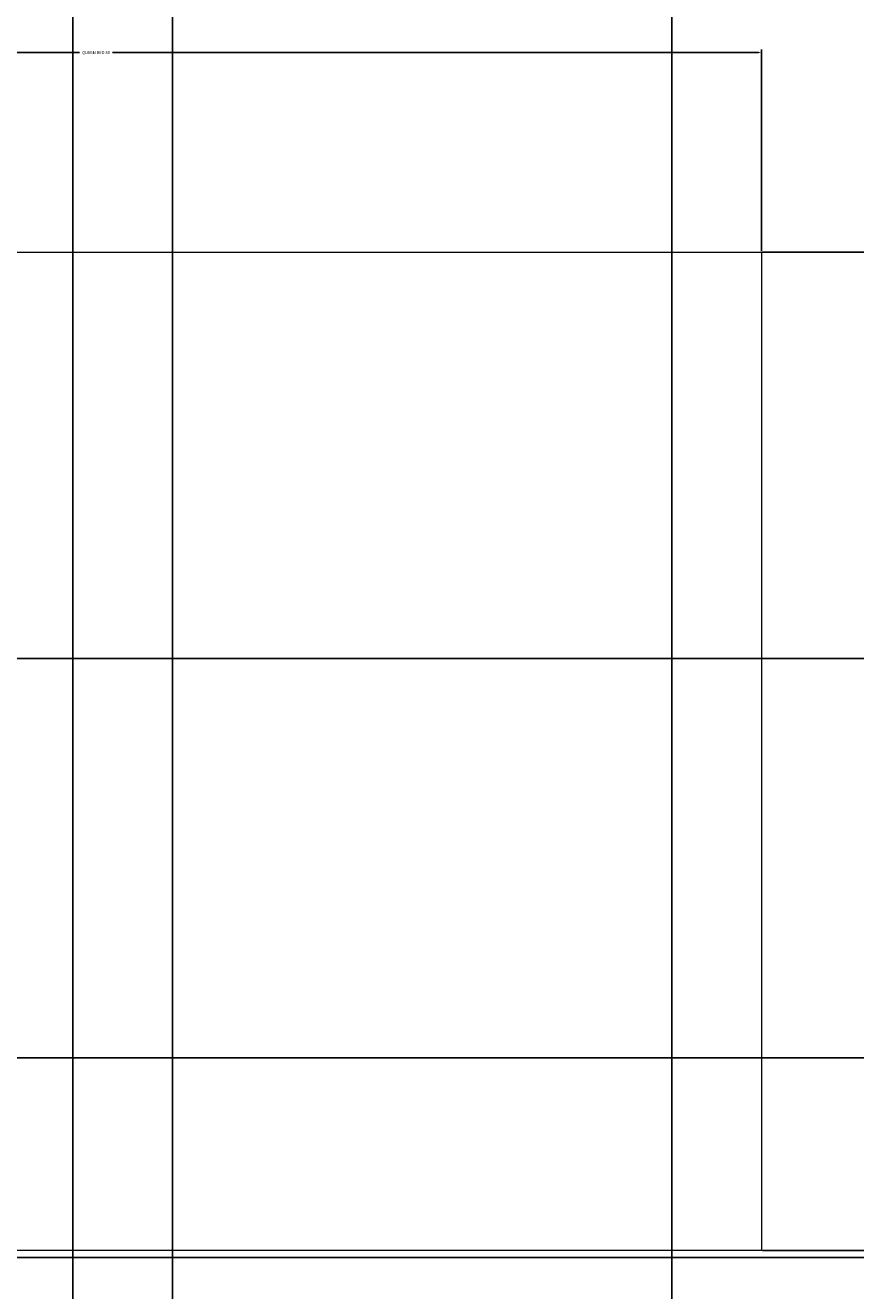
# Model space of a CAD drawing. Units: inches. Extents: x 2231 to 2461, y 2045 to 2455.
# Tile 73 of 95: x 2296 to 2346, y 2333 to 2409. Entities that reach past the tile are written whole.
import ezdxf

# ---------------------------------------------------------------- set-up
doc = ezdxf.new("R2010")
doc.units = ezdxf.units.IN
doc.layers.add('A-ANNO-DIMS', color=2, linetype='Continuous', lineweight=18)
doc.layers.add('A-FURN', color=9, linetype='Continuous', lineweight=18)
doc.styles.get("Standard").update_dxf_attribs({"font": 'arial.ttf'})
doc.dimstyles.get("Standard").update_dxf_attribs({"dimtxt": 0.18, "dimasz": 0.18, "dimexe": 0.18, "dimexo": 0.0625, "dimgap": 0.09, "dimtad": 0, "dimtih": 1, "dimtoh": 1, "dimdec": 4, "dimzin": 0, "dimdsep": 46, "dimtxsty": 'Standard', "dimcen": 0.09, "dimadec": 0, "dimazin": 0, "dimtfac": 1, "dimtdec": 4, "dimtofl": 0, "dimtmove": 0, "dimatfit": 3, "dimfxl": 1, "dimtolj": 1, "dimtzin": 0, "dimarcsym": 0})

# ---------------------------------------------------------------- blocks, each defined once
blk = doc.blocks.new('Bed - Queen')
for p, q in [((0, -80.00003), (0, 0)), ((59.99999, 0), (59.99999, -80.00003)), ((59.99999, -80.00003), (0, -80.00003))]:
    blk.add_line(p, q)
blk = doc.blocks.new('*D19')
at = {"layer": 'A-ANNO-DIMS', "color": 0, "lineweight": -2, "transparency": 16777216}
for p, q in [((2260.188, 2395.316), (2260.188, 2407.433)), ((2260.368, 2407.253), (2299.194, 2407.253)), ((2340.008, 2407.253), (2301.182, 2407.253)), ((2340.188, 2395.316), (2340.188, 2407.433))]:
    blk.add_line(p, q, dxfattribs=at)
at = {"layer": 'A-ANNO-DIMS', "color": 0, "transparency": 16777216}
for points in [[(2260.368, 2407.283), (2260.368, 2407.223), (2260.188, 2407.253)], [(2340.008, 2407.283), (2340.008, 2407.223), (2340.188, 2407.253)]]:
    blk.add_solid(points, dxfattribs=at)
at = {"layer": 'Defpoints', "color": 0, "transparency": 16777216}
for p in [(2260.188, 2407.253), (2260.188, 2395.253), (2340.188, 2395.253)]:
    blk.add_point(p, dxfattribs=at)
at = {"layer": 'A-ANNO-DIMS', "color": 0, "transparency": 16777216, "insert": (2300.188, 2407.253), "char_height": 0.18, "attachment_point": 5}
blk.add_mtext('\\A1;QUEEN BED 80', dxfattribs=at)
blk = doc.blocks.new('*D20')
at = {"layer": 'A-ANNO-DIMS', "color": 0, "lineweight": -2, "transparency": 16777216}
for p, q in [((2340.251, 2395.253), (2352.368, 2395.253)), ((2352.188, 2395.073), (2352.188, 2365.435)), ((2352.188, 2335.433), (2352.188, 2365.071)), ((2340.251, 2335.253), (2352.368, 2335.253))]:
    blk.add_line(p, q, dxfattribs=at)
at = {"layer": 'A-ANNO-DIMS', "color": 0, "transparency": 16777216}
for points in [[(2352.158, 2395.073), (2352.218, 2395.073), (2352.188, 2395.253)], [(2352.158, 2335.433), (2352.218, 2335.433), (2352.188, 2335.253)]]:
    blk.add_solid(points, dxfattribs=at)
at = {"layer": 'Defpoints', "color": 0, "transparency": 16777216}
for p in [(2340.188, 2395.253), (2352.188, 2395.253), (2340.188, 2335.253)]:
    blk.add_point(p, dxfattribs=at)
at = {"layer": 'A-ANNO-DIMS', "color": 0, "transparency": 16777216, "insert": (2352.188, 2365.253), "char_height": 0.18, "attachment_point": 5}
blk.add_mtext('\\A1;60', dxfattribs=at)
blk = doc.blocks.new('*D49')
at = {"layer": 'A-ANNO-DIMS', "color": 0, "lineweight": -2, "transparency": 16777216}
for p, q in [((2298.794, 2182.895), (2298.794, 2454.645)), ((2298.974, 2454.465), (2301.644, 2454.465)), ((2304.614, 2454.465), (2301.943, 2454.465)), ((2304.794, 2182.895), (2304.794, 2454.645))]:
    blk.add_line(p, q, dxfattribs=at)
at = {"layer": 'A-ANNO-DIMS', "color": 0, "transparency": 16777216}
for points in [[(2298.974, 2454.495), (2298.974, 2454.435), (2298.794, 2454.465)], [(2304.614, 2454.495), (2304.614, 2454.435), (2304.794, 2454.465)]]:
    blk.add_solid(points, dxfattribs=at)
at = {"layer": 'Defpoints', "color": 0, "transparency": 16777216}
for p in [(2304.794, 2454.465), (2298.794, 2182.833), (2304.794, 2182.833)]:
    blk.add_point(p, dxfattribs=at)
at = {"layer": 'A-ANNO-DIMS', "color": 0, "transparency": 16777216, "insert": (2301.794, 2454.465), "char_height": 0.18, "attachment_point": 5}
blk.add_mtext('\\A1;6', dxfattribs=at)
blk = doc.blocks.new('*D50')
at = {"layer": 'A-ANNO-DIMS', "color": 0, "lineweight": -2, "transparency": 16777216}
for p, q in [((2304.794, 2182.895), (2304.794, 2454.645)), ((2304.974, 2454.465), (2319.575, 2454.465)), ((2334.614, 2454.465), (2320.012, 2454.465)), ((2334.794, 2182.895), (2334.794, 2454.645))]:
    blk.add_line(p, q, dxfattribs=at)
at = {"layer": 'A-ANNO-DIMS', "color": 0, "transparency": 16777216}
for points in [[(2304.974, 2454.495), (2304.974, 2454.435), (2304.794, 2454.465)], [(2334.614, 2454.495), (2334.614, 2454.435), (2334.794, 2454.465)]]:
    blk.add_solid(points, dxfattribs=at)
at = {"layer": 'Defpoints', "color": 0, "transparency": 16777216}
for p in [(2334.794, 2454.465), (2304.794, 2182.833), (2334.794, 2182.833)]:
    blk.add_point(p, dxfattribs=at)
at = {"layer": 'A-ANNO-DIMS', "color": 0, "transparency": 16777216, "insert": (2319.794, 2454.465), "char_height": 0.18, "attachment_point": 5}
blk.add_mtext('\\A1;30', dxfattribs=at)
blk = doc.blocks.new('*D53')
at = {"layer": 'A-ANNO-DIMS', "color": 0, "lineweight": -2, "transparency": 16777216}
for p, q in [((2372.731, 2346.833), (2230.981, 2346.833)), ((2231.161, 2346.653), (2231.161, 2341.013)), ((2231.161, 2335.013), (2231.161, 2340.652)), ((2372.731, 2334.833), (2230.981, 2334.833))]:
    blk.add_line(p, q, dxfattribs=at)
at = {"layer": 'A-ANNO-DIMS', "color": 0, "transparency": 16777216}
for points in [[(2231.131, 2346.653), (2231.191, 2346.653), (2231.161, 2346.833)], [(2231.131, 2335.013), (2231.191, 2335.013), (2231.161, 2334.833)]]:
    blk.add_solid(points, dxfattribs=at)
at = {"layer": 'Defpoints', "color": 0, "transparency": 16777216}
for p in [(2231.161, 2346.833), (2372.794, 2346.833), (2372.794, 2334.833)]:
    blk.add_point(p, dxfattribs=at)
at = {"layer": 'A-ANNO-DIMS', "color": 0, "transparency": 16777216, "insert": (2231.161, 2340.833), "char_height": 0.18, "attachment_point": 5}
blk.add_mtext('\\A1;12', dxfattribs=at)
blk = doc.blocks.new('*D54')
at = {"layer": 'A-ANNO-DIMS', "color": 0, "lineweight": -2, "transparency": 16777216}
for p, q in [((2372.731, 2370.833), (2230.981, 2370.833)), ((2231.161, 2370.653), (2231.161, 2359.013)), ((2231.161, 2347.013), (2231.161, 2358.652)), ((2372.731, 2346.833), (2230.981, 2346.833))]:
    blk.add_line(p, q, dxfattribs=at)
at = {"layer": 'A-ANNO-DIMS', "color": 0, "transparency": 16777216}
for points in [[(2231.131, 2370.653), (2231.191, 2370.653), (2231.161, 2370.833)], [(2231.131, 2347.013), (2231.191, 2347.013), (2231.161, 2346.833)]]:
    blk.add_solid(points, dxfattribs=at)
at = {"layer": 'Defpoints', "color": 0, "transparency": 16777216}
for p in [(2231.161, 2370.833), (2372.794, 2370.833), (2372.794, 2346.833)]:
    blk.add_point(p, dxfattribs=at)
at = {"layer": 'A-ANNO-DIMS', "color": 0, "transparency": 16777216, "insert": (2231.161, 2358.833), "char_height": 0.18, "attachment_point": 5}
blk.add_mtext('\\A1;24', dxfattribs=at)

msp = doc.modelspace()

# ---------------------------------------------------------------- block references
at = {"layer": 'A-FURN', "rotation": 90}
msp.add_blockref('Bed - Queen', (2260.1881, 2335.2534), dxfattribs=at)

# ---------------------------------------------------------------- dimensions: what is measured, and where the dimension line sits
at = {"layer": 'A-ANNO-DIMS'}
for base, p1, p2, picture, middle in [((2304.7935, 2454.4653), (2298.7935, 2182.8328), (2304.7935, 2182.8328), '*D49', (2301.7935, 2454.4653)), ((2334.7935, 2454.4653), (2304.7935, 2182.8328), (2334.7935, 2182.8328), '*D50', (2319.7935, 2454.4653))]:
    dim = msp.add_linear_dim(base=base, p1=p1, p2=p2, dimstyle='Standard', override={"dimdec": 0, "dimlfac": 1, "dimrnd": 0, "dimzin": 0, "dimdsep": 46, "dimlunit": 2}, dxfattribs=at)
    dim.commit()
    dim.dimension.update_dxf_attribs({"geometry": picture, "text_midpoint": middle})
dim = msp.add_linear_dim(base=(2260.1881, 2407.2534), p1=(2340.1882, 2395.2534), p2=(2260.1881, 2395.2534), angle=180, text='QUEEN BED <>', dimstyle='Standard', override={"dimdec": 0, "dimlfac": 1, "dimrnd": 0, "dimzin": 0, "dimdsep": 46, "dimlunit": 2}, dxfattribs=at)
dim.commit()
dim.dimension.update_dxf_attribs({"geometry": '*D19', "text_midpoint": (2300.1882, 2407.2534)})
for base, p1, p2, picture, middle in [((2352.1882, 2395.2534), (2340.1882, 2335.2534), (2340.1882, 2395.2534), '*D20', (2352.1882, 2365.2534)), ((2231.161, 2370.8328), (2372.7935, 2346.8328), (2372.7935, 2370.8328), '*D54', (2231.161, 2358.8328)), ((2231.161, 2346.8328), (2372.7935, 2334.8328), (2372.7935, 2346.8328), '*D53', (2231.161, 2340.8328))]:
    dim = msp.add_linear_dim(base=base, p1=p1, p2=p2, angle=90, dimstyle='Standard', override={"dimdec": 0, "dimlfac": 1, "dimrnd": 0, "dimzin": 0, "dimdsep": 46, "dimlunit": 2}, dxfattribs=at)
    dim.commit()
    dim.dimension.update_dxf_attribs({"geometry": picture, "text_midpoint": middle})

doc.saveas('drawing.dxf')
